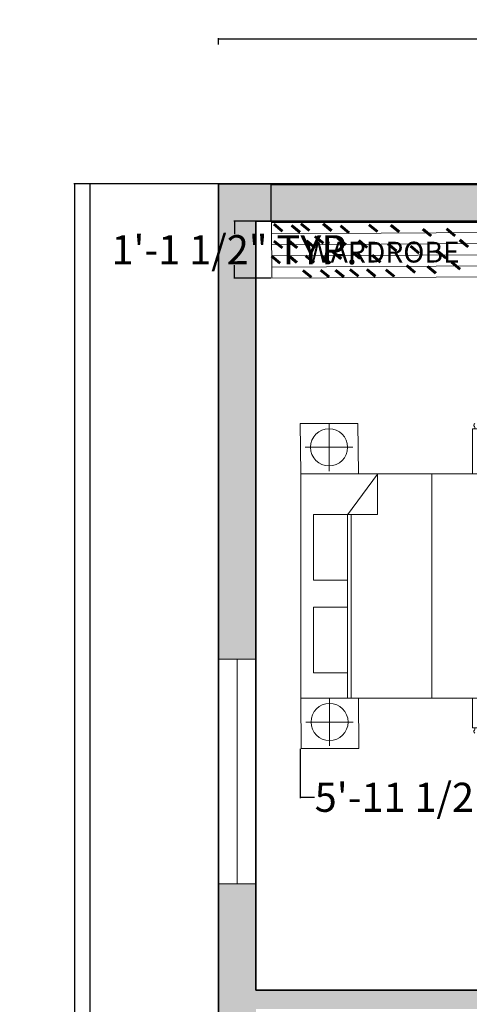
# Model space of a CAD drawing. Units: inches. Extents: x 136 to 672, y -412 to 279.
# Tile 4 of 6: x 136 to 244, y 42 to 279. Entities that reach past the tile are written whole.
import ezdxf

# ---------------------------------------------------------------- set-up
doc = ezdxf.new("R2010")
doc.units = ezdxf.units.IN
doc.header["$MEASUREMENT"] = 0
for name, color, linetype, lineweight in [('A-ANNO-DIMS', 12, 'Continuous', 18), ('A-ANNO-TEXT', 7, 'Continuous', 18), ('A-FLOR-CASE', 252, 'Continuous', 18), ('A-FLOR-CASE-PATT', 9, 'Continuous', 9), ('A-WALL-PATT', 244, 'Continuous', 9), ('furniture', 252, 'Continuous', 18), ('walls', 253, 'Continuous', 35), ('windows', 171, 'Continuous', 18)]:
    doc.layers.add(name, color=color, linetype=linetype, lineweight=lineweight)
doc.styles.get("Standard").update_dxf_attribs({"font": 'arial.ttf'})
doc.dimstyles.get("Standard").update_dxf_attribs({"dimtxt": 7, "dimasz": 0.18, "dimexe": 0.18, "dimexo": 0.0625, "dimgap": 0.09, "dimtad": 0, "dimtih": 1, "dimtoh": 1, "dimzin": 0, "dimdsep": 46, "dimlunit": 3, "dimtxsty": 'Standard', "dimcen": 0.09, "dimadec": 0, "dimazin": 0, "dimtfac": 1, "dimtofl": 0, "dimtmove": 0, "dimatfit": 3, "dimfxl": 1, "dimtolj": 1, "dimtzin": 0, "dimarcsym": 0})

# ---------------------------------------------------------------- blocks, each defined once
blk = doc.blocks.new('CARPET')
at = {"layer": 'furniture'}
for p, q in [((-51.53, -98.11), (-51.53, -55.12)), ((-51.53, -55.12), (-41.27, -55.12)), ((36, -55.12), (51.55, -55.12)), ((51.55, -55.12), (51.55, -98.11)), ((51.55, -98.11), (-51.53, -98.11))]:
    blk.add_line(p, q, dxfattribs=at)
for points, knots in [([(-53.37, -55.99), (-53.22, -55.8), (-52.9, -55.41), (-52.34, -55.8), (-51.89, -56.08), (-51.65, -55.91), (-51.53, -55.83)], [0, 0, 0, 0, 0.653278, 1.290138, 1.740457, 2.114451, 2.114451, 2.114451, 2.114451]), ([(-53.37, -57.26), (-53.22, -57.07), (-52.9, -56.67), (-52.34, -57.07), (-51.89, -57.35), (-51.65, -57.17), (-51.53, -57.1)], [0, 0, 0, 0, 0.653278, 1.290138, 1.740457, 2.114451, 2.114451, 2.114451, 2.114451]), ([(53.37, -55.99), (53.22, -55.8), (52.9, -55.41), (52.34, -55.8), (51.89, -56.08), (51.65, -55.91), (51.53, -55.83)], [0, 0, 0, 0, 0.653278, 1.290138, 1.740457, 2.114451, 2.114451, 2.114451, 2.114451]), ([(53.37, -57.26), (53.22, -57.07), (52.9, -56.67), (52.34, -57.07), (51.89, -57.35), (51.65, -57.17), (51.53, -57.1)], [0, 0, 0, 0, 0.653278, 1.290138, 1.740457, 2.114451, 2.114451, 2.114451, 2.114451]), ([(-53.37, -58.59), (-53.22, -58.4), (-52.9, -58.01), (-52.34, -58.4), (-51.89, -58.68), (-51.65, -58.5), (-51.53, -58.43)], [0, 0, 0, 0, 0.653278, 1.290138, 1.740457, 2.114451, 2.114451, 2.114451, 2.114451]), ([(-53.37, -59.78), (-53.22, -59.58), (-52.9, -59.19), (-52.34, -59.58), (-51.89, -59.86), (-51.65, -59.69), (-51.53, -59.61)], [0, 0, 0, 0, 0.653278, 1.290138, 1.740457, 2.114451, 2.114451, 2.114451, 2.114451]), ([(-53.37, -61.22), (-53.22, -61.02), (-52.9, -60.63), (-52.34, -61.02), (-51.89, -61.3), (-51.65, -61.13), (-51.53, -61.05)], [0, 0, 0, 0, 0.653278, 1.290138, 1.740457, 2.114451, 2.114451, 2.114451, 2.114451]), ([(53.37, -58.59), (53.22, -58.4), (52.9, -58.01), (52.34, -58.4), (51.89, -58.68), (51.65, -58.5), (51.53, -58.43)], [0, 0, 0, 0, 0.653278, 1.290138, 1.740457, 2.114451, 2.114451, 2.114451, 2.114451]), ([(53.37, -59.78), (53.22, -59.58), (52.9, -59.19), (52.34, -59.58), (51.89, -59.86), (51.65, -59.69), (51.53, -59.61)], [0, 0, 0, 0, 0.653278, 1.290138, 1.740457, 2.114451, 2.114451, 2.114451, 2.114451]), ([(53.37, -61.22), (53.22, -61.02), (52.9, -60.63), (52.34, -61.02), (51.89, -61.3), (51.65, -61.13), (51.53, -61.05)], [0, 0, 0, 0, 0.653278, 1.290138, 1.740457, 2.114451, 2.114451, 2.114451, 2.114451]), ([(-53.37, -62.44), (-53.22, -62.25), (-52.9, -61.86), (-52.34, -62.25), (-51.89, -62.53), (-51.65, -62.36), (-51.53, -62.28)], [0, 0, 0, 0, 0.653278, 1.290138, 1.740457, 2.114451, 2.114451, 2.114451, 2.114451]), ([(-53.37, -63.63), (-53.22, -63.43), (-52.9, -63.04), (-52.34, -63.43), (-51.89, -63.72), (-51.65, -63.54), (-51.53, -63.46)], [0, 0, 0, 0, 0.653278, 1.290138, 1.740457, 2.114451, 2.114451, 2.114451, 2.114451]), ([(53.37, -62.44), (53.22, -62.25), (52.9, -61.86), (52.34, -62.25), (51.89, -62.53), (51.65, -62.36), (51.53, -62.28)], [0, 0, 0, 0, 0.653278, 1.290138, 1.740457, 2.114451, 2.114451, 2.114451, 2.114451]), ([(53.37, -63.63), (53.22, -63.43), (52.9, -63.04), (52.34, -63.43), (51.89, -63.72), (51.65, -63.54), (51.53, -63.46)], [0, 0, 0, 0, 0.653278, 1.290138, 1.740457, 2.114451, 2.114451, 2.114451, 2.114451]), ([(-53.37, -65.07), (-53.22, -64.87), (-52.9, -64.48), (-52.34, -64.87), (-51.89, -65.15), (-51.65, -64.98), (-51.53, -64.9)], [0, 0, 0, 0, 0.653278, 1.290138, 1.740457, 2.114451, 2.114451, 2.114451, 2.114451]), ([(-53.37, -66.76), (-53.22, -66.56), (-52.9, -66.17), (-52.34, -66.56), (-51.89, -66.84), (-51.65, -66.67), (-51.53, -66.59)], [0, 0, 0, 0, 0.653278, 1.290138, 1.740457, 2.114451, 2.114451, 2.114451, 2.114451]), ([(-53.37, -68.2), (-53.22, -68), (-52.9, -67.61), (-52.34, -68), (-51.89, -68.28), (-51.65, -68.11), (-51.53, -68.03)], [0, 0, 0, 0, 0.653278, 1.290138, 1.740457, 2.114451, 2.114451, 2.114451, 2.114451]), ([(53.37, -65.07), (53.22, -64.87), (52.9, -64.48), (52.34, -64.87), (51.89, -65.15), (51.65, -64.98), (51.53, -64.9)], [0, 0, 0, 0, 0.653278, 1.290138, 1.740457, 2.114451, 2.114451, 2.114451, 2.114451]), ([(53.37, -66.76), (53.22, -66.56), (52.9, -66.17), (52.34, -66.56), (51.89, -66.84), (51.65, -66.67), (51.53, -66.59)], [0, 0, 0, 0, 0.653278, 1.290138, 1.740457, 2.114451, 2.114451, 2.114451, 2.114451]), ([(53.37, -68.2), (53.22, -68), (52.9, -67.61), (52.34, -68), (51.89, -68.28), (51.65, -68.11), (51.53, -68.03)], [0, 0, 0, 0, 0.653278, 1.290138, 1.740457, 2.114451, 2.114451, 2.114451, 2.114451]), ([(-53.37, -69.53), (-53.22, -69.33), (-52.9, -68.94), (-52.34, -69.33), (-51.89, -69.61), (-51.65, -69.44), (-51.53, -69.36)], [0, 0, 0, 0, 0.653278, 1.290138, 1.740457, 2.114451, 2.114451, 2.114451, 2.114451]), ([(-53.37, -70.79), (-53.22, -70.6), (-52.9, -70.21), (-52.34, -70.6), (-51.89, -70.88), (-51.65, -70.7), (-51.53, -70.63)], [0, 0, 0, 0, 0.653278, 1.290138, 1.740457, 2.114451, 2.114451, 2.114451, 2.114451]), ([(53.37, -69.53), (53.22, -69.33), (52.9, -68.94), (52.34, -69.33), (51.89, -69.61), (51.65, -69.44), (51.53, -69.36)], [0, 0, 0, 0, 0.653278, 1.290138, 1.740457, 2.114451, 2.114451, 2.114451, 2.114451]), ([(53.37, -70.79), (53.22, -70.6), (52.9, -70.21), (52.34, -70.6), (51.89, -70.88), (51.65, -70.7), (51.53, -70.63)], [0, 0, 0, 0, 0.653278, 1.290138, 1.740457, 2.114451, 2.114451, 2.114451, 2.114451]), ([(-53.37, -72.12), (-53.22, -71.93), (-52.9, -71.54), (-52.34, -71.93), (-51.89, -72.21), (-51.65, -72.04), (-51.53, -71.96)], [0, 0, 0, 0, 0.653278, 1.290138, 1.740457, 2.114451, 2.114451, 2.114451, 2.114451]), ([(-53.37, -73.31), (-53.22, -73.11), (-52.9, -72.72), (-52.34, -73.11), (-51.89, -73.4), (-51.65, -73.22), (-51.53, -73.14)], [0, 0, 0, 0, 0.653278, 1.290138, 1.740457, 2.114451, 2.114451, 2.114451, 2.114451]), ([(-53.37, -74.75), (-53.22, -74.55), (-52.9, -74.16), (-52.34, -74.55), (-51.89, -74.83), (-51.65, -74.66), (-51.53, -74.58)], [0, 0, 0, 0, 0.653278, 1.290138, 1.740457, 2.114451, 2.114451, 2.114451, 2.114451]), ([(53.37, -72.12), (53.22, -71.93), (52.9, -71.54), (52.34, -71.93), (51.89, -72.21), (51.65, -72.04), (51.53, -71.96)], [0, 0, 0, 0, 0.653278, 1.290138, 1.740457, 2.114451, 2.114451, 2.114451, 2.114451]), ([(53.37, -73.31), (53.22, -73.11), (52.9, -72.72), (52.34, -73.11), (51.89, -73.4), (51.65, -73.22), (51.53, -73.14)], [0, 0, 0, 0, 0.653278, 1.290138, 1.740457, 2.114451, 2.114451, 2.114451, 2.114451]), ([(53.37, -74.75), (53.22, -74.55), (52.9, -74.16), (52.34, -74.55), (51.89, -74.83), (51.65, -74.66), (51.53, -74.58)], [0, 0, 0, 0, 0.653278, 1.290138, 1.740457, 2.114451, 2.114451, 2.114451, 2.114451]), ([(-53.37, -75.98), (-53.22, -75.78), (-52.9, -75.39), (-52.34, -75.78), (-51.89, -76.06), (-51.65, -75.89), (-51.53, -75.81)], [0, 0, 0, 0, 0.653278, 1.290138, 1.740457, 2.114451, 2.114451, 2.114451, 2.114451]), ([(-53.37, -77.16), (-53.22, -76.96), (-52.9, -76.57), (-52.34, -76.96), (-51.89, -77.25), (-51.65, -77.07), (-51.53, -76.99)], [0, 0, 0, 0, 0.653278, 1.290138, 1.740457, 2.114451, 2.114451, 2.114451, 2.114451]), ([(53.37, -75.98), (53.22, -75.78), (52.9, -75.39), (52.34, -75.78), (51.89, -76.06), (51.65, -75.89), (51.53, -75.81)], [0, 0, 0, 0, 0.653278, 1.290138, 1.740457, 2.114451, 2.114451, 2.114451, 2.114451]), ([(53.37, -77.16), (53.22, -76.96), (52.9, -76.57), (52.34, -76.96), (51.89, -77.25), (51.65, -77.07), (51.53, -76.99)], [0, 0, 0, 0, 0.653278, 1.290138, 1.740457, 2.114451, 2.114451, 2.114451, 2.114451]), ([(-53.37, -78.6), (-53.22, -78.4), (-52.9, -78.01), (-52.34, -78.4), (-51.89, -78.68), (-51.65, -78.51), (-51.53, -78.43)], [0, 0, 0, 0, 0.653278, 1.290138, 1.740457, 2.114451, 2.114451, 2.114451, 2.114451]), ([(-53.37, -80.29), (-53.22, -80.09), (-52.9, -79.7), (-52.34, -80.09), (-51.89, -80.37), (-51.65, -80.2), (-51.53, -80.12)], [0, 0, 0, 0, 0.653278, 1.290138, 1.740457, 2.114451, 2.114451, 2.114451, 2.114451]), ([(-53.37, -81.73), (-53.22, -81.53), (-52.9, -81.14), (-52.34, -81.53), (-51.89, -81.81), (-51.65, -81.64), (-51.53, -81.56)], [0, 0, 0, 0, 0.653278, 1.290138, 1.740457, 2.114451, 2.114451, 2.114451, 2.114451]), ([(53.37, -78.6), (53.22, -78.4), (52.9, -78.01), (52.34, -78.4), (51.89, -78.68), (51.65, -78.51), (51.53, -78.43)], [0, 0, 0, 0, 0.653278, 1.290138, 1.740457, 2.114451, 2.114451, 2.114451, 2.114451]), ([(53.37, -80.29), (53.22, -80.09), (52.9, -79.7), (52.34, -80.09), (51.89, -80.37), (51.65, -80.2), (51.53, -80.12)], [0, 0, 0, 0, 0.653278, 1.290138, 1.740457, 2.114451, 2.114451, 2.114451, 2.114451]), ([(53.37, -81.73), (53.22, -81.53), (52.9, -81.14), (52.34, -81.53), (51.89, -81.81), (51.65, -81.64), (51.53, -81.56)], [0, 0, 0, 0, 0.653278, 1.290138, 1.740457, 2.114451, 2.114451, 2.114451, 2.114451]), ([(-53.37, -83.06), (-53.22, -82.86), (-52.9, -82.47), (-52.34, -82.86), (-51.89, -83.14), (-51.65, -82.97), (-51.53, -82.89)], [0, 0, 0, 0, 0.653278, 1.290138, 1.740457, 2.114451, 2.114451, 2.114451, 2.114451]), ([(-53.37, -84.18), (-53.22, -83.99), (-52.9, -83.6), (-52.34, -83.99), (-51.89, -84.27), (-51.65, -84.09), (-51.53, -84.02)], [0, 0, 0, 0, 0.653278, 1.290138, 1.740457, 2.114451, 2.114451, 2.114451, 2.114451]), ([(53.37, -83.06), (53.22, -82.86), (52.9, -82.47), (52.34, -82.86), (51.89, -83.14), (51.65, -82.97), (51.53, -82.89)], [0, 0, 0, 0, 0.653278, 1.290138, 1.740457, 2.114451, 2.114451, 2.114451, 2.114451]), ([(53.37, -84.18), (53.22, -83.99), (52.9, -83.6), (52.34, -83.99), (51.89, -84.27), (51.65, -84.09), (51.53, -84.02)], [0, 0, 0, 0, 0.653278, 1.290138, 1.740457, 2.114451, 2.114451, 2.114451, 2.114451]), ([(-53.37, -85.51), (-53.22, -85.32), (-52.9, -84.93), (-52.34, -85.32), (-51.89, -85.6), (-51.65, -85.42), (-51.53, -85.35)], [0, 0, 0, 0, 0.653278, 1.290138, 1.740457, 2.114451, 2.114451, 2.114451, 2.114451]), ([(-53.37, -86.7), (-53.22, -86.5), (-52.9, -86.11), (-52.34, -86.5), (-51.89, -86.78), (-51.65, -86.61), (-51.53, -86.53)], [0, 0, 0, 0, 0.653278, 1.290138, 1.740457, 2.114451, 2.114451, 2.114451, 2.114451]), ([(-53.37, -88.14), (-53.22, -87.94), (-52.9, -87.55), (-52.34, -87.94), (-51.89, -88.22), (-51.65, -88.05), (-51.53, -87.97)], [0, 0, 0, 0, 0.653278, 1.290138, 1.740457, 2.114451, 2.114451, 2.114451, 2.114451]), ([(53.37, -85.51), (53.22, -85.32), (52.9, -84.93), (52.34, -85.32), (51.89, -85.6), (51.65, -85.42), (51.53, -85.35)], [0, 0, 0, 0, 0.653278, 1.290138, 1.740457, 2.114451, 2.114451, 2.114451, 2.114451]), ([(53.37, -86.7), (53.22, -86.5), (52.9, -86.11), (52.34, -86.5), (51.89, -86.78), (51.65, -86.61), (51.53, -86.53)], [0, 0, 0, 0, 0.653278, 1.290138, 1.740457, 2.114451, 2.114451, 2.114451, 2.114451]), ([(53.37, -88.14), (53.22, -87.94), (52.9, -87.55), (52.34, -87.94), (51.89, -88.22), (51.65, -88.05), (51.53, -87.97)], [0, 0, 0, 0, 0.653278, 1.290138, 1.740457, 2.114451, 2.114451, 2.114451, 2.114451]), ([(-53.37, -89.36), (-53.22, -89.17), (-52.9, -88.78), (-52.34, -89.17), (-51.89, -89.45), (-51.65, -89.28), (-51.53, -89.2)], [0, 0, 0, 0, 0.653278, 1.290138, 1.740457, 2.114451, 2.114451, 2.114451, 2.114451]), ([(-53.37, -90.55), (-53.22, -90.35), (-52.9, -89.96), (-52.34, -90.35), (-51.89, -90.64), (-51.65, -90.46), (-51.53, -90.38)], [0, 0, 0, 0, 0.653278, 1.290138, 1.740457, 2.114451, 2.114451, 2.114451, 2.114451]), ([(-53.37, -91.99), (-53.22, -91.79), (-52.9, -91.4), (-52.34, -91.79), (-51.89, -92.07), (-51.65, -91.9), (-51.53, -91.82)], [0, 0, 0, 0, 0.653278, 1.290138, 1.740457, 2.114451, 2.114451, 2.114451, 2.114451]), ([(53.37, -89.36), (53.22, -89.17), (52.9, -88.78), (52.34, -89.17), (51.89, -89.45), (51.65, -89.28), (51.53, -89.2)], [0, 0, 0, 0, 0.653278, 1.290138, 1.740457, 2.114451, 2.114451, 2.114451, 2.114451]), ([(53.37, -90.55), (53.22, -90.35), (52.9, -89.96), (52.34, -90.35), (51.9, -90.63), (51.66, -90.47), (51.55, -90.4)], [0, 0, 0, 0, 0.653278, 1.290138, 1.740457, 2.0926, 2.0926, 2.0926, 2.0926]), ([(53.37, -91.99), (53.22, -91.79), (52.9, -91.4), (52.34, -91.79), (51.9, -92.07), (51.66, -91.91), (51.55, -91.83)], [0, 0, 0, 0, 0.653278, 1.290138, 1.740457, 2.0926, 2.0926, 2.0926, 2.0926]), ([(-53.37, -92.69), (-53.22, -92.48), (-52.9, -92.08), (-52.35, -92.49), (-51.89, -92.77), (-51.65, -92.6), (-51.53, -92.52)], [0, 0, 0, 0, 0.663904, 1.307406, 1.757725, 2.131719, 2.131719, 2.131719, 2.131719]), ([(-53.37, -93.61), (-53.22, -93.42), (-52.9, -93.03), (-52.34, -93.42), (-51.89, -93.7), (-51.65, -93.52), (-51.53, -93.45)], [0, 0, 0, 0, 0.653278, 1.290138, 1.740457, 2.114451, 2.114451, 2.114451, 2.114451]), ([(-53.37, -94.55), (-53.22, -94.35), (-52.9, -93.96), (-52.34, -94.35), (-51.89, -94.63), (-51.65, -94.46), (-51.53, -94.38)], [0, 0, 0, 0, 0.653278, 1.290138, 1.740457, 2.114451, 2.114451, 2.114451, 2.114451]), ([(-53.37, -95.05), (-53.22, -94.85), (-52.9, -94.46), (-52.34, -94.85), (-51.89, -95.14), (-51.65, -94.96), (-51.53, -94.88)], [0, 0, 0, 0, 0.653278, 1.290138, 1.740457, 2.114451, 2.114451, 2.114451, 2.114451]), ([(53.37, -92.69), (53.22, -92.49), (52.9, -92.09), (52.34, -92.49), (51.9, -92.77), (51.66, -92.61), (51.55, -92.53)], [0, 0, 0, 0, 0.656792, 1.295826, 1.746145, 2.098292, 2.098292, 2.098292, 2.098292]), ([(53.37, -93.66), (53.22, -93.46), (52.9, -93.07), (52.34, -93.46), (51.9, -93.74), (51.66, -93.58), (51.55, -93.5)], [0, 0, 0, 0, 0.653278, 1.290138, 1.740457, 2.0926, 2.0926, 2.0926, 2.0926]), ([(53.37, -94.59), (53.22, -94.4), (52.9, -94.01), (52.34, -94.4), (51.9, -94.68), (51.66, -94.51), (51.55, -94.44)], [0, 0, 0, 0, 0.653278, 1.290138, 1.740457, 2.0926, 2.0926, 2.0926, 2.0926]), ([(53.37, -95.1), (53.22, -94.9), (52.9, -94.51), (52.34, -94.9), (51.9, -95.18), (51.66, -95.02), (51.55, -94.94)], [0, 0, 0, 0, 0.653278, 1.290138, 1.740457, 2.0926, 2.0926, 2.0926, 2.0926]), ([(-53.37, -95.73), (-53.22, -95.54), (-52.9, -95.15), (-52.34, -95.54), (-51.89, -95.82), (-51.65, -95.65), (-51.53, -95.57)], [0, 0, 0, 0, 0.653278, 1.290138, 1.740457, 2.114451, 2.114451, 2.114451, 2.114451]), ([(-53.37, -96.38), (-53.22, -96.18), (-52.9, -95.79), (-52.34, -96.18), (-51.89, -96.47), (-51.65, -96.29), (-51.53, -96.21)], [0, 0, 0, 0, 0.653278, 1.290138, 1.740457, 2.114451, 2.114451, 2.114451, 2.114451]), ([(-53.37, -97.17), (-53.22, -96.98), (-52.9, -96.59), (-52.34, -96.98), (-51.89, -97.26), (-51.65, -97.08), (-51.53, -97.01)], [0, 0, 0, 0, 0.653278, 1.290138, 1.740457, 2.114451, 2.114451, 2.114451, 2.114451]), ([(-53.37, -97.99), (-53.22, -97.79), (-52.9, -97.4), (-52.34, -97.79), (-51.89, -98.08), (-51.65, -97.9), (-51.53, -97.82)], [0, 0, 0, 0, 0.653278, 1.290138, 1.740457, 2.114451, 2.114451, 2.114451, 2.114451]), ([(53.37, -95.78), (53.22, -95.58), (52.9, -95.19), (52.34, -95.58), (51.89, -95.86), (51.65, -95.69), (51.53, -95.61)], [0, 0, 0, 0, 0.653278, 1.290138, 1.740457, 2.114451, 2.114451, 2.114451, 2.114451]), ([(53.37, -96.43), (53.22, -96.23), (52.9, -95.84), (52.34, -96.23), (51.89, -96.51), (51.65, -96.34), (51.53, -96.26)], [0, 0, 0, 0, 0.653278, 1.290138, 1.740457, 2.114451, 2.114451, 2.114451, 2.114451]), ([(53.37, -97.22), (53.22, -97.02), (52.9, -96.63), (52.34, -97.02), (51.89, -97.3), (51.65, -97.13), (51.53, -97.05)], [0, 0, 0, 0, 0.653278, 1.290138, 1.740457, 2.114451, 2.114451, 2.114451, 2.114451]), ([(53.37, -97.99), (53.22, -97.79), (52.9, -97.4), (52.34, -97.79), (51.89, -98.08), (51.65, -97.9), (51.53, -97.82)], [0, 0, 0, 0, 0.653278, 1.290138, 1.740457, 2.114451, 2.114451, 2.114451, 2.114451])]:
    blk.add_open_spline(points, degree=3, knots=knots, dxfattribs=at)
blk = doc.blocks.new('A$C58D270C6')
at = {"layer": 'furniture'}
for p, q in [((9.09, 124.13), (9.09, 108.87)), ((1.46, 116.5), (16.73, 116.5)), ((14.97, 94.84), (24.62, 107.92)), ((24.62, 94.93), (24.62, 107.92)), ((42.08, 108), (42.08, 36)), ((14.97, 94.93), (24.62, 94.93)), ((14.97, 94.84), (14.97, 36)), ((16.22, 94.93), (16.22, 36)), ((9.25, 36), (9.25, 20.74)), ((1.62, 28.37), (16.88, 28.37))]:
    blk.add_line(p, q, dxfattribs=at)
for points in [[(18.5, 108), (18.34, 124.13), (-0.16, 124.13), (0, 108)], [(0, 108), (77.91, 108), (77.91, 36), (0, 36)], [(4.09, 94.93), (14.97, 94.93), (14.97, 73.83), (4.09, 73.83)], [(4.09, 65.23), (14.97, 65.23), (14.97, 44.13), (4.09, 44.13)], [(18.65, 19.87), (18.5, 36), (0, 36), (0.16, 19.87)]]:
    blk.add_lwpolyline(points, close=True, dxfattribs=at)
for centre in [(9.09, 116.5), (9.25, 28.37)]:
    blk.add_circle(centre, 5.95, dxfattribs=at)
at = {"layer": 'furniture', "xscale": 0.9312884925094044, "yscale": 0.9312884925094044, "zscale": 0.9312884925094044, "rotation": 90}
blk.add_blockref('CARPET', (3.79, 74.47), dxfattribs=at)
blk = doc.blocks.new('*D18')
at = {"layer": 'A-ANNO-DIMS', "color": 0, "lineweight": -2, "transparency": 16777216}
for p, q in [((183.46, 273.1), (183.46, 274.63)), ((183.64, 274.45), (387.44, 274.45)), ((603.28, 274.45), (399.49, 274.45)), ((603.46, 273.1), (603.46, 274.63))]:
    blk.add_line(p, q, dxfattribs=at)
at = {"layer": 'A-ANNO-DIMS', "color": 0, "transparency": 16777216}
for points in [[(183.64, 274.48), (183.64, 274.42), (183.46, 274.45)], [(603.28, 274.48), (603.28, 274.42), (603.46, 274.45)]]:
    blk.add_solid(points, dxfattribs=at)
at = {"layer": 'Defpoints', "color": 0, "transparency": 16777216}
for p in [(183.46, 273.04), (603.46, 274.45), (603.46, 273.04)]:
    blk.add_point(p, dxfattribs=at)
at = {"layer": 'A-ANNO-DIMS', "color": 0, "transparency": 16777216, "insert": (393.46, 274.45), "char_height": 7, "attachment_point": 5}
blk.add_mtext("\\A1;35'", dxfattribs=at)
blk = doc.blocks.new('*D19')
at = {"layer": 'A-ANNO-DIMS', "color": 0, "lineweight": -2, "transparency": 16777216}
for p, q in [((152.44, 239.56), (152.7, 239.56)), ((152.52, 239.38), (152.52, -56.77)), ((152.52, -360.26), (152.52, -64.1)), ((152.44, -360.44), (152.7, -360.44))]:
    blk.add_line(p, q, dxfattribs=at)
at = {"layer": 'A-ANNO-DIMS', "color": 0, "transparency": 16777216}
for points in [[(152.49, 239.38), (152.55, 239.38), (152.52, 239.56)], [(152.49, -360.26), (152.55, -360.26), (152.52, -360.44)]]:
    blk.add_solid(points, dxfattribs=at)
at = {"layer": 'Defpoints', "color": 0, "transparency": 16777216}
for p in [(152.38, 239.56), (152.38, -360.44), (152.52, -360.44)]:
    blk.add_point(p, dxfattribs=at)
at = {"layer": 'A-ANNO-DIMS', "color": 0, "transparency": 16777216, "insert": (152.52, -60.44), "char_height": 7, "attachment_point": 5}
blk.add_mtext("\\A1;50'", dxfattribs=at)
blk = doc.blocks.new('WIN-54')
for p, q in [((0, 54.05), (9, 54.05)), ((0, 0), (0, 54.05)), ((0, 54.05), (4.5, 54.05)), ((4.5, 54.05), (4.5, 0)), ((9, 54.05), (9, 0)), ((9, 0), (0, 0))]:
    blk.add_line(p, q)
blk = doc.blocks.new('WARDROBE-FRAME')
for p, q in [((0, 13.37), (58.88, 13.37)), ((0.05, 13.37), (0.13, 0)), ((58.95, 0.34), (58.88, 13.71)), ((0.02, 10.69), (58.89, 11.04)), ((0.03, 8.02), (58.91, 8.36)), ((0.05, 5.35), (58.92, 5.69)), ((0.06, 2.67), (58.94, 3.02)), ((0.08, 0), (58.95, 0.34))]:
    blk.add_line(p, q)
blk = doc.blocks.new('*D28')
at = {"layer": 'A-ANNO-DIMS', "color": 0, "lineweight": -2, "transparency": 16777216}
for p, q in [((203.15, 103.66), (203.15, 91.81)), ((274.61, 103.66), (274.61, 91.81)), ((203.33, 91.99), (206.58, 91.99)), ((274.43, 91.99), (271.18, 91.99))]:
    blk.add_line(p, q, dxfattribs=at)
at = {"layer": 'A-ANNO-DIMS', "color": 0, "transparency": 16777216}
for points in [[(203.33, 92.02), (203.33, 91.96), (203.15, 91.99)], [(274.43, 92.02), (274.43, 91.96), (274.61, 91.99)]]:
    blk.add_solid(points, dxfattribs=at)
at = {"layer": 'Defpoints', "color": 0, "transparency": 16777216}
for p in [(203.15, 103.72), (274.61, 103.72), (274.61, 91.99)]:
    blk.add_point(p, dxfattribs=at)
at = {"layer": 'A-ANNO-DIMS', "color": 0, "transparency": 16777216, "insert": (238.88, 91.99), "char_height": 7, "attachment_point": 5}
blk.add_mtext('\\A1;5\'-11 1/2" TYP.', dxfattribs=at)
blk = doc.blocks.new('*D29')
at = {"layer": 'A-ANNO-DIMS', "color": 0, "lineweight": -2, "transparency": 16777216}
for p, q in [((196.15, 230.63), (196.15, 239.59)), ((196.33, 239.41), (254.92, 239.41)), ((255.1, 230.63), (255.1, 239.59)), ((255.1, 239.41), (255.28, 239.41))]:
    blk.add_line(p, q, dxfattribs=at)
at = {"layer": 'A-ANNO-DIMS', "color": 0, "transparency": 16777216}
for points in [[(196.33, 239.44), (196.33, 239.38), (196.15, 239.41)], [(254.92, 239.44), (254.92, 239.38), (255.1, 239.41)]]:
    blk.add_solid(points, dxfattribs=at)
at = {"layer": 'Defpoints', "color": 0, "transparency": 16777216}
for p in [(255.1, 239.41), (196.15, 230.56), (255.1, 230.56)]:
    blk.add_point(p, dxfattribs=at)
at = {"layer": 'A-ANNO-DIMS', "color": 0, "transparency": 16777216, "insert": (309.72, 239.41), "char_height": 7, "attachment_point": 5}
blk.add_mtext('\\A1;WARDROBE 4\'-11" TYP.', dxfattribs=at)
blk = doc.blocks.new('*D30')
at = {"layer": 'A-ANNO-DIMS', "color": 0, "lineweight": -2, "transparency": 16777216}
for p, q in [((196.09, 230.56), (187.13, 230.56)), ((187.31, 230.38), (187.31, 227.42)), ((187.31, 217.03), (187.31, 220)), ((196.09, 216.85), (187.13, 216.85))]:
    blk.add_line(p, q, dxfattribs=at)
at = {"layer": 'A-ANNO-DIMS', "color": 0, "transparency": 16777216}
for points in [[(187.28, 230.38), (187.34, 230.38), (187.31, 230.56)], [(187.28, 217.03), (187.34, 217.03), (187.31, 216.85)]]:
    blk.add_solid(points, dxfattribs=at)
at = {"layer": 'Defpoints', "color": 0, "transparency": 16777216}
for p in [(187.31, 230.56), (196.15, 230.56), (196.15, 216.85)]:
    blk.add_point(p, dxfattribs=at)
at = {"layer": 'A-ANNO-DIMS', "color": 0, "transparency": 16777216, "insert": (187.31, 223.71), "char_height": 7, "attachment_point": 5}
blk.add_mtext('\\A1;1\'-1 1/2" TYP.', dxfattribs=at)
blk = doc.blocks.new('*D56')
at = {"layer": 'A-ANNO-DIMS', "color": 0, "lineweight": -2, "transparency": 16777216}
for p, q in [((183.4, 239.56), (148.63, 239.56)), ((148.81, 239.38), (148.81, -62.84)), ((148.81, -372.4), (148.81, -70.17)), ((219.39, -372.58), (148.63, -372.58))]:
    blk.add_line(p, q, dxfattribs=at)
at = {"layer": 'A-ANNO-DIMS', "color": 0, "transparency": 16777216}
for points in [[(148.78, 239.38), (148.84, 239.38), (148.81, 239.56)], [(148.78, -372.4), (148.84, -372.4), (148.81, -372.58)]]:
    blk.add_solid(points, dxfattribs=at)
at = {"layer": 'Defpoints', "color": 0, "transparency": 16777216}
for p in [(183.46, 239.56), (148.81, -372.58), (219.45, -372.58)]:
    blk.add_point(p, dxfattribs=at)
at = {"layer": 'A-ANNO-DIMS', "color": 0, "transparency": 16777216, "insert": (148.81, -66.51), "char_height": 7, "attachment_point": 5}
blk.add_mtext('\\A1;51\'-0"', dxfattribs=at)

msp = doc.modelspace()

# ---------------------------------------------------------------- hatches: boundary and pattern name
at = {"layer": 'A-FLOR-CASE-PATT'}
h = msp.add_hatch(dxfattribs=at)
h.set_pattern_fill('ANSI31', color=256, scale=0.8474926, angle=95.46701, style=0)
h.paths.add_polyline_path([(198.969, 228.356), (196.972, 230.004), (196.698, 229.673), (198.695, 228.025)])
h = msp.add_hatch(dxfattribs=at)
h.set_pattern_fill('ANSI31', color=256, scale=0.847474, angle=95.467, style=0)
h.paths.add_polyline_path([(205.467, 228.479), (203.47, 230.127), (203.196, 229.795), (205.193, 228.147)])
h = msp.add_hatch(dxfattribs=at)
h.set_pattern_fill('ANSI31', color=256, scale=0.847436, angle=95.467, style=0)
h.paths.add_polyline_path([(210.796, 228.458), (208.799, 230.106), (208.526, 229.774), (210.522, 228.126)])
h = msp.add_hatch(dxfattribs=at)
h.set_pattern_fill('ANSI31', color=256, scale=0.8473843, angle=95.46701, style=0)
h.paths.add_polyline_path([(221.851, 228.237), (219.854, 229.885), (219.581, 229.553), (221.577, 227.905)])
h = msp.add_hatch(dxfattribs=at)
h.set_pattern_fill('ANSI31', color=256, scale=0.8476002, angle=95.46701, style=0)
h.paths.add_polyline_path([(227.083, 228.145), (225.086, 229.793), (224.813, 229.461), (226.81, 227.813)])
h = msp.add_hatch(dxfattribs=at)
h.set_pattern_fill('ANSI31', color=256, scale=0.847587, angle=95.467, style=0)
h.paths.add_polyline_path([(203.212, 228.058), (201.215, 229.706), (200.942, 229.374), (202.938, 227.726)])
h = msp.add_hatch(dxfattribs=at)
h.set_pattern_fill('ANSI31', color=256, scale=0.8476313, angle=95.46701, style=0)
h.paths.add_polyline_path([(215.018, 227.951), (213.021, 229.599), (212.748, 229.267), (214.744, 227.619)])
h = msp.add_hatch(dxfattribs=at)
h.set_pattern_fill('ANSI31', color=256, scale=0.847406, angle=95.467, style=0)
h.paths.add_polyline_path([(234.782, 227.189), (232.785, 228.837), (232.511, 228.506), (234.508, 226.858)])
h = msp.add_hatch(dxfattribs=at)
h.set_pattern_fill('ANSI31', color=256, scale=0.8476247, angle=95.46701, style=0)
h.paths.add_polyline_path([(240.532, 227.223), (238.535, 228.871), (238.261, 228.539), (240.258, 226.891)])
h = msp.add_hatch(dxfattribs=at)
h.set_pattern_fill('ANSI31', color=256, scale=0.8476432, angle=95.46701, style=0)
h.paths.add_polyline_path([(198.967, 224.306), (196.97, 225.954), (196.696, 225.623), (198.693, 223.975)])
h = msp.add_hatch(dxfattribs=at)
h.set_pattern_fill('ANSI31', color=256, scale=0.8475317, angle=95.46701, style=0)
h.paths.add_polyline_path([(202.541, 224.327), (200.544, 225.975), (200.271, 225.644), (202.268, 223.995)])
h = msp.add_hatch(dxfattribs=at)
h.set_pattern_fill('ANSI31', color=256, scale=0.8475266, angle=95.46701, style=0)
h.paths.add_polyline_path([(206.835, 224.352), (204.839, 226), (204.565, 225.669), (206.562, 224.021)])
h = msp.add_hatch(dxfattribs=at)
h.set_pattern_fill('ANSI31', color=256, scale=0.8474898, angle=95.46701, style=0)
h.paths.add_polyline_path([(208.83, 225.436), (206.833, 227.084), (206.559, 226.753), (208.556, 225.105)])
h = msp.add_hatch(dxfattribs=at)
h.set_pattern_fill('ANSI31', color=256, scale=0.8474864, angle=95.46701, style=0)
h.paths.add_polyline_path([(214.249, 225.083), (212.252, 226.731), (211.979, 226.399), (213.975, 224.751)])
h = msp.add_hatch(dxfattribs=at)
h.set_pattern_fill('ANSI31', color=256, scale=0.8474845, angle=95.46701, style=0)
h.paths.add_polyline_path([(219.371, 224.426), (217.374, 226.074), (217.101, 225.742), (219.097, 224.094)])
h = msp.add_hatch(dxfattribs=at)
h.set_pattern_fill('ANSI31', color=256, scale=0.8473727, angle=95.46701, style=0)
h.paths.add_polyline_path([(226.415, 223.641), (224.418, 225.289), (224.144, 224.957), (226.141, 223.309)])
h = msp.add_hatch(dxfattribs=at)
h.set_pattern_fill('ANSI31', color=256, scale=0.8475184, angle=95.46701, style=0)
h.paths.add_polyline_path([(243.684, 224.568), (241.687, 226.216), (241.414, 225.885), (243.41, 224.237)])
h = msp.add_hatch(dxfattribs=at)
h.set_pattern_fill('ANSI31', color=256, scale=0.847425, angle=95.467, style=0)
h.paths.add_polyline_path([(213.134, 221.716), (211.138, 223.364), (210.864, 223.032), (212.861, 221.384)])
h = msp.add_hatch(dxfattribs=at)
h.set_pattern_fill('ANSI31', color=256, scale=0.8476336, angle=95.46701, style=0)
h.paths.add_polyline_path([(217.715, 221.743), (215.718, 223.391), (215.444, 223.059), (217.441, 221.411)])
h = msp.add_hatch(dxfattribs=at)
h.set_pattern_fill('ANSI31', color=256, scale=0.8474992, angle=95.46701, style=0)
h.paths.add_polyline_path([(231.854, 223.059), (229.857, 224.707), (229.583, 224.375), (231.58, 222.727)])
h = msp.add_hatch(dxfattribs=at)
h.set_pattern_fill('ANSI31', color=256, scale=0.847621, angle=95.467, style=0)
h.paths.add_polyline_path([(238.368, 221.864), (236.371, 223.512), (236.097, 223.18), (238.094, 221.532)])
h = msp.add_hatch(dxfattribs=at)
h.set_pattern_fill('ANSI31', color=256, scale=0.847658, angle=95.467, style=0)
h.paths.add_polyline_path([(198.395, 220.664), (196.398, 222.312), (196.124, 221.98), (198.121, 220.332)])
h = msp.add_hatch(dxfattribs=at)
h.set_pattern_fill('ANSI31', color=256, scale=0.8475074, angle=95.46701, style=0)
h.paths.add_polyline_path([(202.456, 220.815), (200.459, 222.463), (200.185, 222.132), (202.182, 220.484)])
h = msp.add_hatch(dxfattribs=at)
h.set_pattern_fill('ANSI31', color=256, scale=0.8473717, angle=95.46701, style=0)
h.paths.add_polyline_path([(206.6, 220.766), (204.604, 222.414), (204.33, 222.082), (206.327, 220.434)])
h = msp.add_hatch(dxfattribs=at)
h.set_pattern_fill('ANSI31', color=256, scale=0.8476324, angle=95.46701, style=0)
h.paths.add_polyline_path([(210.528, 220.667), (208.531, 222.315), (208.257, 221.983), (210.254, 220.335)])
h = msp.add_hatch(dxfattribs=at)
h.set_pattern_fill('ANSI31', color=256, scale=0.84741, angle=95.467, style=0)
h.paths.add_polyline_path([(222.58, 220.918), (220.583, 222.566), (220.309, 222.234), (222.306, 220.586)])
h = msp.add_hatch(dxfattribs=at)
h.set_pattern_fill('ANSI31', color=256, scale=0.847587, angle=95.467, style=0)
h.paths.add_polyline_path([(241.729, 219.21), (239.732, 220.858), (239.459, 220.527), (241.455, 218.879)])
h = msp.add_hatch(dxfattribs=at)
h.set_pattern_fill('ANSI31', color=256, scale=0.847536, angle=95.467, style=0)
h.paths.add_polyline_path([(205.945, 217.262), (203.948, 218.91), (203.675, 218.578), (205.671, 216.93)])
h = msp.add_hatch(dxfattribs=at)
h.set_pattern_fill('ANSI31', color=256, scale=0.8475436, angle=95.46701, style=0)
h.paths.add_polyline_path([(210.21, 217.317), (208.213, 218.965), (207.94, 218.633), (209.936, 216.985)])
h = msp.add_hatch(dxfattribs=at)
h.set_pattern_fill('ANSI31', color=256, scale=0.8474087, angle=95.46701, style=0)
h.paths.add_polyline_path([(213.77, 217.338), (211.773, 218.986), (211.499, 218.655), (213.496, 217.006)])
h = msp.add_hatch(dxfattribs=at)
h.set_pattern_fill('ANSI31', color=256, scale=0.847451, angle=95.467, style=0)
h.paths.add_polyline_path([(217.279, 217.484), (215.282, 219.132), (215.008, 218.8), (217.005, 217.152)])
h = msp.add_hatch(dxfattribs=at)
h.set_pattern_fill('ANSI31', color=256, scale=0.8475362, angle=95.46701, style=0)
h.paths.add_polyline_path([(221.336, 217.472), (219.34, 219.12), (219.066, 218.788), (221.063, 217.14)])
h = msp.add_hatch(dxfattribs=at)
h.set_pattern_fill('ANSI31', color=256, scale=0.8475664, angle=95.46701, style=0)
h.paths.add_polyline_path([(225.911, 217.419), (223.914, 219.068), (223.64, 218.736), (225.637, 217.088)])
h = msp.add_hatch(dxfattribs=at)
h.set_pattern_fill('ANSI31', color=256, scale=0.8473777, angle=95.46701, style=0)
h.paths.add_polyline_path([(230.9, 218.431), (228.903, 220.079), (228.63, 219.747), (230.627, 218.099)])
h = msp.add_hatch(dxfattribs=at)
h.set_pattern_fill('ANSI31', color=256, scale=0.8475595, angle=95.46701, style=0)
h.paths.add_polyline_path([(235.929, 218.215), (233.932, 219.863), (233.658, 219.531), (235.655, 217.883)])
at = {"layer": 'A-WALL-PATT'}
h = msp.add_hatch(color=256, dxfattribs=at)
h.dxf.hatch_style = 1
h.paths.add_polyline_path([(255.026, 239.565), (183.463, 239.565), (183.463, 125.252), (187.963, 125.252), (192.463, 125.252), (192.463, 230.565), (255.024, 230.565), (255.025, 235.065)])
h.paths.add_polyline_path([(369.355, 239.565), (332.259, 239.565), (332.259, 230.565), (342.463, 230.565), (342.463, 104.521), (346.963, 104.521), (346.963, 230.565), (369.355, 230.565), (369.355, 235.065)])
h.paths.add_polyline_path([(603.463, 239.565), (385.627, 239.565), (385.627, 230.565), (406.963, 230.565), (406.963, 134.565), (371.802, 134.565), (371.802, 130.065), (406.963, 130.065), (406.963, 45.565), (346.963, 45.565), (346.963, 69.395), (342.463, 69.395), (342.463, 45.565), (332.733, 45.565), (332.733, 41.065), (416.87, 41.065), (416.87, 45.565), (411.463, 45.565), (411.463, 230.565), (594.463, 230.565), (594.463, 199.893), (598.963, 199.893), (603.463, 199.893)])
h.paths.add_polyline_path([(603.463, 145.845), (594.463, 145.845), (594.463, 98.065), (524.374, 98.065), (512.275, 97.948), (512.275, 98.065), (484.021, 98.065), (484.021, 93.565), (505.963, 93.565), (594.463, 93.565), (594.463, 80.073), (598.963, 80.073), (603.463, 80.073)], flags=17)
h.paths.add_polyline_path([(457.963, 98.065), (453.463, 98.065), (453.463, 41.065), (594.463, 41.065), (594.463, -67.933), (603.463, -67.933), (603.463, 63.801), (594.463, 63.801), (594.463, 45.565), (510.463, 45.565), (510.463, 65.243), (505.963, 65.243), (505.963, 45.565), (457.963, 45.565)])
h.paths.add_polyline_path([(192.463, 71.205), (183.463, 71.205), (183.463, 25.824), (192.463, 25.824), (192.463, 41.065), (296.463, 41.065), (296.463, 24.884), (300.963, 24.884), (300.963, 45.565), (192.463, 45.565)])
h.paths.add_polyline_path([(300.963, -6.935), (296.463, -6.935), (192.463, -6.935), (192.463, -11.435), (300.963, -11.435)])
h.paths.add_polyline_path([(192.463, 8.674), (183.463, 8.674), (183.463, -44.733), (187.963, -44.733), (192.463, -44.733)])
h.paths.add_polyline_path([(235.886, -349.935), (192.463, -349.935), (192.463, -358.935), (235.886, -358.935)])
h.paths.add_polyline_path([(345.463, -316.935), (361.986, -316.935), (361.986, -307.935), (340.963, -307.935), (340.963, -229.935), (356.354, -229.935), (356.354, -225.435), (336.463, -225.435), (336.463, -349.935), (300.655, -349.935), (300.655, -358.935), (345.463, -358.935)])
h.paths.add_polyline_path([(407.452, -307.935), (403.463, -307.935), (403.463, -225.435), (382.286, -225.435), (382.286, -229.935), (398.963, -229.935), (398.963, -307.935), (379.137, -307.935), (379.137, -316.935), (407.452, -316.935)])
h.paths.add_polyline_path([(470.463, -284.28), (461.463, -284.28), (461.463, -307.935), (461.463, -316.935), (470.463, -316.935)])
h.paths.add_polyline_path([(470.463, -234.435), (480.349, -234.435), (480.349, -225.435), (461.463, -225.435), (461.463, -245.135), (470.463, -245.135)])
h.paths.add_polyline_path([(603.463, -121.943), (594.463, -121.943), (594.463, -225.435), (574.368, -225.435), (574.368, -234.435), (603.463, -234.435)])
h.paths.add_polyline_path([(340.963, -75.678), (336.463, -75.678), (336.463, -168.061), (340.963, -168.061)])
h.paths.add_polyline_path([(468.637, 59.14), (510.671, 59.14), (510.671, 68.331), (468.637, 68.331)], flags=25)
h.paths.add_polyline_path([(192.463, -208.04), (183.463, -208.04), (183.463, -360.435), (192.463, -360.435)])
h.paths.add_polyline_path([(183.463, -153.992), (192.463, -153.992), (192.463, -98.781), (183.463, -98.781)])

# ---------------------------------------------------------------- linework, layer by layer
at = {"layer": 'A-FLOR-CASE'}
msp.add_line((196.149, 230.22), (196.202, 230.22), dxfattribs=at)
at = {"layer": 'walls'}
for p, q in [((183.463, 239.565), (603.463, 239.565)), ((183.463, -360.435), (183.463, 239.565)), ((192.463, 230.565), (342.463, 230.565)), ((192.463, 45.565), (192.463, 230.565)), ((192.463, 45.565), (300.963, 45.565))]:
    msp.add_line(p, q, dxfattribs=at)

# ---------------------------------------------------------------- block references
at = {"layer": 'A-FLOR-CASE'}
msp.add_blockref('WARDROBE-FRAME', (196.149, 216.854), dxfattribs=at)
at = {"layer": 'furniture', "xscale": 0.7498206902034922, "yscale": 0.7498206902034922, "zscale": 0.7498206902034922}
msp.add_blockref('A$C58D270C6', (203.262, 88.822), dxfattribs=at)
at = {"layer": 'windows'}
msp.add_blockref('WIN-54', (183.463, 71.205), dxfattribs=at)

# ---------------------------------------------------------------- texts
at = {"layer": 'A-ANNO-TEXT'}
msp.add_text('WARDROBE', height=5, dxfattribs=at).set_placement((204.468, 220.629))

# ---------------------------------------------------------------- dimensions: what is measured, and where the dimension line sits
at = {"layer": 'A-ANNO-DIMS'}
dim = msp.add_linear_dim(base=(603.463, 274.45), p1=(183.463, 273.039), p2=(603.463, 273.039), dimstyle='Standard', override={"dimclrd": 0, "dimclre": 0, "dimclrt": 0}, dxfattribs=at)
dim.commit()
dim.dimension.update_dxf_attribs({"geometry": '*D18', "text_midpoint": (393.463, 274.45)})
for base, p1, p2, text, picture, middle in [((255.103, 239.408), (196.149, 230.565), (255.103, 230.565), 'WARDROBE <> TYP.', '*D29', (309.723, 239.408)), ((274.614, 91.988), (203.145, 103.72), (274.614, 103.72), '<> TYP.', '*D28', (238.88, 91.988))]:
    dim = msp.add_linear_dim(base=base, p1=p1, p2=p2, text=text, dimstyle='Standard', override={"dimdec": 1, "dimlfac": 1, "dimrnd": 0, "dimzin": 1, "dimdsep": 46, "dimlunit": 4, "dimfrac": 2}, dxfattribs=at)
    dim.commit()
    dim.dimension.update_dxf_attribs({"geometry": picture, "text_midpoint": middle})
for base, p1, p2, override, picture, middle in [((148.813, -372.578), (183.463, 239.565), (219.455, -372.578), {"dimdec": 1, "dimlfac": 1, "dimrnd": 0, "dimzin": 1, "dimdsep": 46, "dimlunit": 4, "dimfrac": 2}, '*D56', (148.813, -66.506)), ((152.519, -360.435), (152.38, 239.565), (152.38, -360.435), {"dimclrd": 0, "dimclre": 0, "dimclrt": 0}, '*D19', (152.519, -60.435))]:
    dim = msp.add_linear_dim(base=base, p1=p1, p2=p2, angle=90, dimstyle='Standard', override=override, dxfattribs=at)
    dim.commit()
    dim.dimension.update_dxf_attribs({"geometry": picture, "text_midpoint": middle})
dim = msp.add_linear_dim(base=(187.306, 230.565), p1=(196.149, 216.854), p2=(196.149, 230.565), angle=90, text='<> TYP.', dimstyle='Standard', override={"dimdec": 1, "dimlfac": 1, "dimrnd": 0, "dimzin": 1, "dimdsep": 46, "dimlunit": 4, "dimfrac": 2}, dxfattribs=at)
dim.commit()
dim.dimension.update_dxf_attribs({"geometry": '*D30', "text_midpoint": (187.306, 223.709)})

doc.saveas('drawing.dxf')
